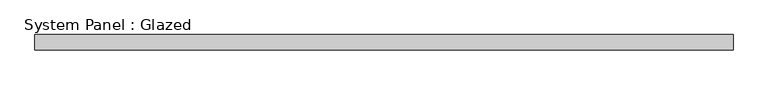
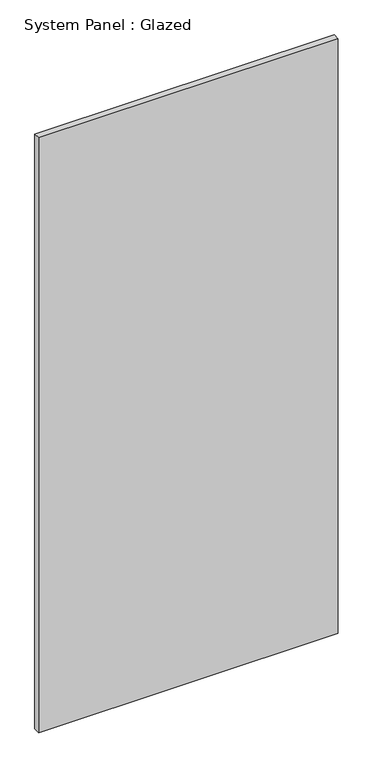
"""IFC4 building model written with IfcOpenShell, lengths in millimetres: plate geometry, System Panel : Glazed."""

from ifc_helpers import new_model, si_unit, origin, origin_with_axes, place, context, project, spatial, polyline, outline, extrude, source, transform, mapped, element, save


def system_panel_glazed_d770e50e(model_context):
    return source(origin(), model_context, "Body", "SweptSolid", [
        extrude(outline(polyline([(571.7712628, 24.5), (-571.7712628, 24.5), (-571.7712628, 49.5), (571.7712628, 49.5), (571.7712628, 24.5)])), origin_with_axes(), (0.0, 0.0, 1.0), 2400.0),
    ])


if __name__ == "__main__":
    model = new_model("IFC4")
    model_context = context("Model", 3, world=origin())
    ifc_project = project(units=[si_unit("LENGTHUNIT", "METRE", prefix="MILLI")], contexts=[model_context])
    site = spatial("IfcSite", under=ifc_project)
    building = spatial("IfcBuilding", under=site)
    placement = place(None, origin())
    system_panel_glazed_shape = system_panel_glazed_d770e50e(model_context)
    element("IfcPlate", 1, ObjectType="System Panel : Glazed", at=placement, inside=building, context=model_context, shape_type="MappedRepresentation", body=[
        mapped(system_panel_glazed_shape, transform((0.0, 0.0, 0.0), x_axis=(1.0, 0.0, 0.0), y_axis=(0.0, 1.0, 0.0), z_axis=(0.0, 0.0, 1.0))),
    ])
    save(model, "model.ifc")

# Revit data of these elements
# Type "System Panel : Glazed"
#   Keynote = "H11"
#   Construction Type Id = "GSP4R"
#   Analytic Construction = "1/8 in Pilkington single glazing"
#   Visual Light Transmittance = 0.9
#   Solar Heat Gain Coefficient = 0.86
#   Heat Transfer Coefficient (U) = 6.7069 W/(m²·K)
#   Define Thermal Properties by = 1
# Element 1 (IfcPlate, "System Panel : Glazed")
#   Materials on its faces: "Glass"
# Materials
#   "Glass": class "Glass", colour RGB 0 128 192, transparency 0.9, Description = "Soda Lime Glass", Cost = 0
